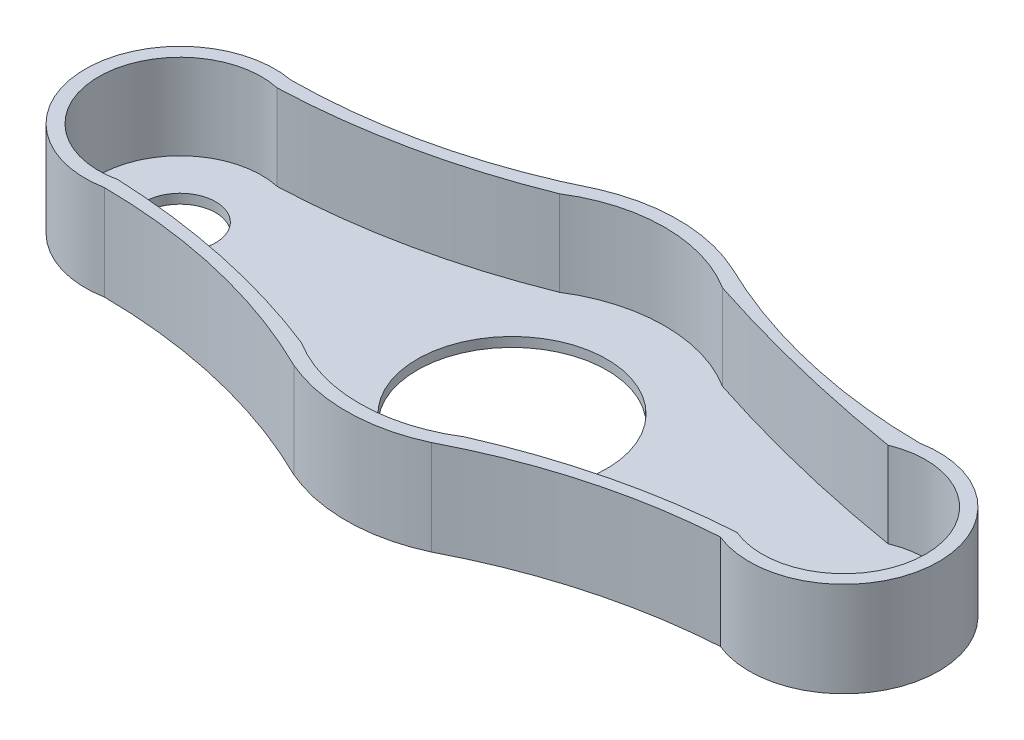
ISO-10303-21;
HEADER;
FILE_DESCRIPTION(('STEP AP214'),'2;1');
FILE_NAME('part.step','',(''),(''),'','','');
FILE_SCHEMA(('AUTOMOTIVE_DESIGN { 1 0 10303 214 1 1 1 1 }'));
ENDSEC;
DATA;
#1=APPLICATION_CONTEXT('core data for automotive mechanical design processes');
#2=APPLICATION_PROTOCOL_DEFINITION('international standard','automotive_design',2000,#1);
#3=PRODUCT_CONTEXT('',#1,'mechanical');
#4=PRODUCT('Part','Part','',(#3));
#5=PRODUCT_RELATED_PRODUCT_CATEGORY('part','',(#4));
#6=PRODUCT_DEFINITION_FORMATION('','',#4);
#7=PRODUCT_DEFINITION_CONTEXT('part definition',#1,'design');
#8=PRODUCT_DEFINITION('design','',#6,#7);
#9=PRODUCT_DEFINITION_SHAPE('','',#8);
#10=(LENGTH_UNIT() NAMED_UNIT(*) SI_UNIT(.MILLI.,.METRE.));
#11=(NAMED_UNIT(*) PLANE_ANGLE_UNIT() SI_UNIT($,.RADIAN.));
#12=(NAMED_UNIT(*) SI_UNIT($,.STERADIAN.) SOLID_ANGLE_UNIT());
#13=UNCERTAINTY_MEASURE_WITH_UNIT(LENGTH_MEASURE(1.E-05),#10,'distance_accuracy_value','');
#14=(GEOMETRIC_REPRESENTATION_CONTEXT(3) GLOBAL_UNCERTAINTY_ASSIGNED_CONTEXT((#13)) GLOBAL_UNIT_ASSIGNED_CONTEXT((#10,
#11,#12)) REPRESENTATION_CONTEXT('',''));
#15=CARTESIAN_POINT('',(0.,0.,0.));
#16=DIRECTION('',(0.,0.,1.));
#17=DIRECTION('',(1.,0.,0.));
#18=AXIS2_PLACEMENT_3D('',#15,#16,#17);
#19=CARTESIAN_POINT('',(-3.70941284252284,20.,0.));
#20=DIRECTION('',(0.,-1.,0.));
#21=DIRECTION('',(0.,0.,-1.));
#22=AXIS2_PLACEMENT_3D('',#19,#20,#21);
#23=CYLINDRICAL_SURFACE('',#22,7.5);
#24=CARTESIAN_POINT('',(-3.70941284252284,0.,0.));
#25=DIRECTION('',(0.,1.,0.));
#26=DIRECTION('',(0.,0.,1.));
#27=AXIS2_PLACEMENT_3D('',#24,#25,#26);
#28=CIRCLE('',#27,7.5);
#29=CARTESIAN_POINT('',(-3.70941284252284,0.,7.5));
#30=VERTEX_POINT('',#29);
#31=EDGE_CURVE('E197',#30,#30,#28,.T.);
#32=ORIENTED_EDGE('',*,*,#31,.F.);
#33=EDGE_LOOP('',(#32));
#34=FACE_BOUND('',#33,.T.);
#35=CARTESIAN_POINT('',(-3.70941284252284,2.,0.));
#36=DIRECTION('',(0.,1.,0.));
#37=DIRECTION('',(0.,0.,1.));
#38=AXIS2_PLACEMENT_3D('',#35,#36,#37);
#39=CIRCLE('',#38,7.5);
#40=CARTESIAN_POINT('',(-3.70941284252284,2.,7.5));
#41=VERTEX_POINT('',#40);
#42=EDGE_CURVE('E193',#41,#41,#39,.T.);
#43=ORIENTED_EDGE('',*,*,#42,.T.);
#44=EDGE_LOOP('',(#43));
#45=FACE_BOUND('',#44,.T.);
#46=ADVANCED_FACE('F41',(#34,#45),#23,.F.);
#47=CARTESIAN_POINT('',(136.290587157477,20.,0.));
#48=DIRECTION('',(0.,-1.,0.));
#49=DIRECTION('',(0.,0.,-1.));
#50=AXIS2_PLACEMENT_3D('',#47,#48,#49);
#51=CYLINDRICAL_SURFACE('',#50,7.50000000000001);
#52=CARTESIAN_POINT('',(136.290587157477,0.,0.));
#53=DIRECTION('',(0.,1.,0.));
#54=DIRECTION('',(0.,0.,1.));
#55=AXIS2_PLACEMENT_3D('',#52,#53,#54);
#56=CIRCLE('',#55,7.50000000000001);
#57=CARTESIAN_POINT('',(136.290587157477,0.,7.50000000000001));
#58=VERTEX_POINT('',#57);
#59=EDGE_CURVE('E192',#58,#58,#56,.T.);
#60=ORIENTED_EDGE('',*,*,#59,.F.);
#61=EDGE_LOOP('',(#60));
#62=FACE_BOUND('',#61,.T.);
#63=CARTESIAN_POINT('',(136.290587157477,2.,0.));
#64=DIRECTION('',(0.,1.,0.));
#65=DIRECTION('',(0.,0.,1.));
#66=AXIS2_PLACEMENT_3D('',#63,#64,#65);
#67=CIRCLE('',#66,7.50000000000001);
#68=CARTESIAN_POINT('',(136.290587157477,2.,7.50000000000001));
#69=VERTEX_POINT('',#68);
#70=EDGE_CURVE('E225',#69,#69,#67,.T.);
#71=ORIENTED_EDGE('',*,*,#70,.T.);
#72=EDGE_LOOP('',(#71));
#73=FACE_BOUND('',#72,.T.);
#74=ADVANCED_FACE('F210',(#62,#73),#51,.F.);
#75=CARTESIAN_POINT('',(66.2905871574772,20.,0.));
#76=DIRECTION('',(0.,-1.,0.));
#77=DIRECTION('',(0.,0.,-1.));
#78=AXIS2_PLACEMENT_3D('',#75,#76,#77);
#79=CYLINDRICAL_SURFACE('',#78,20.);
#80=CARTESIAN_POINT('',(66.2905871574772,0.,0.));
#81=DIRECTION('',(0.,1.,0.));
#82=DIRECTION('',(0.,0.,1.));
#83=AXIS2_PLACEMENT_3D('',#80,#81,#82);
#84=CIRCLE('',#83,20.);
#85=CARTESIAN_POINT('',(66.2905871574772,0.,20.));
#86=VERTEX_POINT('',#85);
#87=EDGE_CURVE('E189',#86,#86,#84,.T.);
#88=ORIENTED_EDGE('',*,*,#87,.F.);
#89=EDGE_LOOP('',(#88));
#90=FACE_BOUND('',#89,.T.);
#91=CARTESIAN_POINT('',(66.2905871574772,2.,0.));
#92=DIRECTION('',(0.,1.,0.));
#93=DIRECTION('',(0.,0.,1.));
#94=AXIS2_PLACEMENT_3D('',#91,#92,#93);
#95=CIRCLE('',#94,20.);
#96=CARTESIAN_POINT('',(66.2905871574772,2.,20.));
#97=VERTEX_POINT('',#96);
#98=EDGE_CURVE('E44',#97,#97,#95,.T.);
#99=ORIENTED_EDGE('',*,*,#98,.T.);
#100=EDGE_LOOP('',(#99));
#101=FACE_BOUND('',#100,.T.);
#102=ADVANCED_FACE('F43',(#90,#101),#79,.F.);
#103=CARTESIAN_POINT('',(133.534659461397,20.,-139.649207998908));
#104=DIRECTION('',(0.,-1.,0.));
#105=DIRECTION('',(0.,0.,-1.));
#106=AXIS2_PLACEMENT_3D('',#103,#104,#105);
#107=CYLINDRICAL_SURFACE('',#106,120.);
#108=CARTESIAN_POINT('',(133.534659461397,0.,-139.649207998908));
#109=DIRECTION('',(0.,1.,0.));
#110=DIRECTION('',(0.,0.,1.));
#111=AXIS2_PLACEMENT_3D('',#108,#109,#110);
#112=CIRCLE('',#111,120.);
#113=CARTESIAN_POINT('',(81.0387041699493,0.,-31.7410309313738));
#114=VERTEX_POINT('',#113);
#115=CARTESIAN_POINT('',(132.581174314954,0.,-19.6529961167178));
#116=VERTEX_POINT('',#115);
#117=EDGE_CURVE('E168',#114,#116,#112,.T.);
#118=ORIENTED_EDGE('',*,*,#117,.F.);
#119=DIRECTION('',(0.,-1.,0.));
#120=VECTOR('',#119,1.);
#121=CARTESIAN_POINT('',(81.0387041699493,20.,-31.7410309313738));
#122=LINE('',#121,#120);
#123=CARTESIAN_POINT('',(81.0387041699493,20.,-31.7410309313738));
#124=VERTEX_POINT('',#123);
#125=EDGE_CURVE('E11',#124,#114,#122,.T.);
#126=ORIENTED_EDGE('',*,*,#125,.F.);
#127=CARTESIAN_POINT('',(133.534659461397,20.,-139.649207998908));
#128=DIRECTION('',(0.,1.,0.));
#129=DIRECTION('',(0.,0.,1.));
#130=AXIS2_PLACEMENT_3D('',#127,#128,#129);
#131=CIRCLE('',#130,120.);
#132=CARTESIAN_POINT('',(132.581174314954,20.,-19.6529961167178));
#133=VERTEX_POINT('',#132);
#134=EDGE_CURVE('E190',#124,#133,#131,.T.);
#135=ORIENTED_EDGE('',*,*,#134,.T.);
#136=DIRECTION('',(0.,-1.,0.));
#137=VECTOR('',#136,1.);
#138=CARTESIAN_POINT('',(132.581174314954,20.,-19.6529961167178));
#139=LINE('',#138,#137);
#140=EDGE_CURVE('E98',#133,#116,#139,.T.);
#141=ORIENTED_EDGE('',*,*,#140,.T.);
#142=EDGE_LOOP('',(#118,#126,#135,#141));
#143=FACE_BOUND('',#142,.T.);
#144=ADVANCED_FACE('F200',(#143),#107,.F.);
#145=CARTESIAN_POINT('',(66.2905871574772,20.,0.));
#146=DIRECTION('',(0.,-1.,0.));
#147=DIRECTION('',(0.,0.,-1.));
#148=AXIS2_PLACEMENT_3D('',#145,#146,#147);
#149=CYLINDRICAL_SURFACE('',#148,35.);
#150=CARTESIAN_POINT('',(66.2905871574772,0.,0.));
#151=DIRECTION('',(0.,1.,0.));
#152=DIRECTION('',(0.,0.,1.));
#153=AXIS2_PLACEMENT_3D('',#150,#151,#152);
#154=CIRCLE('',#153,35.);
#155=CARTESIAN_POINT('',(52.4479221513952,0.,-32.1462381240697));
#156=VERTEX_POINT('',#155);
#157=EDGE_CURVE('E167',#114,#156,#154,.T.);
#158=ORIENTED_EDGE('',*,*,#157,.T.);
#159=DIRECTION('',(0.,-1.,0.));
#160=VECTOR('',#159,1.);
#161=CARTESIAN_POINT('',(52.4479221513952,20.,-32.1462381240697));
#162=LINE('',#161,#160);
#163=CARTESIAN_POINT('',(52.4479221513952,20.,-32.1462381240697));
#164=VERTEX_POINT('',#163);
#165=EDGE_CURVE('E49',#164,#156,#162,.T.);
#166=ORIENTED_EDGE('',*,*,#165,.F.);
#167=CARTESIAN_POINT('',(66.2905871574772,20.,0.));
#168=DIRECTION('',(0.,1.,0.));
#169=DIRECTION('',(0.,0.,1.));
#170=AXIS2_PLACEMENT_3D('',#167,#168,#169);
#171=CIRCLE('',#170,35.);
#172=EDGE_CURVE('E228',#124,#164,#171,.T.);
#173=ORIENTED_EDGE('',*,*,#172,.F.);
#174=ORIENTED_EDGE('',*,*,#125,.T.);
#175=EDGE_LOOP('',(#158,#166,#173,#174));
#176=FACE_BOUND('',#175,.T.);
#177=ADVANCED_FACE('F170',(#176),#149,.T.);
#178=CARTESIAN_POINT('',(-0.871658411644109,20.,-139.649830290013));
#179=DIRECTION('',(0.,-1.,0.));
#180=DIRECTION('',(0.,0.,-1.));
#181=AXIS2_PLACEMENT_3D('',#178,#179,#180);
#182=CYLINDRICAL_SURFACE('',#181,120.);
#183=CARTESIAN_POINT('',(-0.871658411644109,0.,-139.649830290013));
#184=DIRECTION('',(0.,1.,0.));
#185=DIRECTION('',(0.,0.,1.));
#186=AXIS2_PLACEMENT_3D('',#183,#184,#185);
#187=CIRCLE('',#186,120.);
#188=CARTESIAN_POINT('',(0.,0.,-19.6529961167178));
#189=VERTEX_POINT('',#188);
#190=EDGE_CURVE('E161',#189,#156,#187,.T.);
#191=ORIENTED_EDGE('',*,*,#190,.F.);
#192=DIRECTION('',(0.,-1.,0.));
#193=VECTOR('',#192,1.);
#194=CARTESIAN_POINT('',(0.,20.,-19.6529961167178));
#195=LINE('',#194,#193);
#196=CARTESIAN_POINT('',(0.,20.,-19.6529961167178));
#197=VERTEX_POINT('',#196);
#198=EDGE_CURVE('E155',#197,#189,#195,.T.);
#199=ORIENTED_EDGE('',*,*,#198,.F.);
#200=CARTESIAN_POINT('',(-0.871658411644109,20.,-139.649830290013));
#201=DIRECTION('',(0.,1.,0.));
#202=DIRECTION('',(0.,0.,1.));
#203=AXIS2_PLACEMENT_3D('',#200,#201,#202);
#204=CIRCLE('',#203,120.);
#205=EDGE_CURVE('E162',#197,#164,#204,.T.);
#206=ORIENTED_EDGE('',*,*,#205,.T.);
#207=ORIENTED_EDGE('',*,*,#165,.T.);
#208=EDGE_LOOP('',(#191,#199,#206,#207));
#209=FACE_BOUND('',#208,.T.);
#210=ADVANCED_FACE('F157',(#209),#182,.F.);
#211=CARTESIAN_POINT('',(-3.70941284252284,20.,0.));
#212=DIRECTION('',(0.,-1.,0.));
#213=DIRECTION('',(0.,0.,-1.));
#214=AXIS2_PLACEMENT_3D('',#211,#212,#213);
#215=CYLINDRICAL_SURFACE('',#214,20.);
#216=CARTESIAN_POINT('',(-3.70941284252284,0.,0.));
#217=DIRECTION('',(0.,1.,0.));
#218=DIRECTION('',(0.,0.,1.));
#219=AXIS2_PLACEMENT_3D('',#216,#217,#218);
#220=CIRCLE('',#219,20.);
#221=CARTESIAN_POINT('',(0.,0.,19.6529961167178));
#222=VERTEX_POINT('',#221);
#223=EDGE_CURVE('E174',#189,#222,#220,.T.);
#224=ORIENTED_EDGE('',*,*,#223,.T.);
#225=DIRECTION('',(0.,-1.,0.));
#226=VECTOR('',#225,1.);
#227=CARTESIAN_POINT('',(0.,20.,19.6529961167178));
#228=LINE('',#227,#226);
#229=CARTESIAN_POINT('',(0.,20.,19.6529961167178));
#230=VERTEX_POINT('',#229);
#231=EDGE_CURVE('E144',#230,#222,#228,.T.);
#232=ORIENTED_EDGE('',*,*,#231,.F.);
#233=CARTESIAN_POINT('',(-3.70941284252284,20.,0.));
#234=DIRECTION('',(0.,1.,0.));
#235=DIRECTION('',(0.,0.,1.));
#236=AXIS2_PLACEMENT_3D('',#233,#234,#235);
#237=CIRCLE('',#236,20.);
#238=EDGE_CURVE('E235',#197,#230,#237,.T.);
#239=ORIENTED_EDGE('',*,*,#238,.F.);
#240=ORIENTED_EDGE('',*,*,#198,.T.);
#241=EDGE_LOOP('',(#224,#232,#239,#240));
#242=FACE_BOUND('',#241,.T.);
#243=ADVANCED_FACE('F240',(#242),#215,.T.);
#244=CARTESIAN_POINT('',(-0.871658411644109,20.,139.649830290013));
#245=DIRECTION('',(0.,-1.,0.));
#246=DIRECTION('',(0.,0.,-1.));
#247=AXIS2_PLACEMENT_3D('',#244,#245,#246);
#248=CYLINDRICAL_SURFACE('',#247,120.);
#249=CARTESIAN_POINT('',(-0.871658411644109,0.,139.649830290013));
#250=DIRECTION('',(0.,1.,0.));
#251=DIRECTION('',(0.,0.,1.));
#252=AXIS2_PLACEMENT_3D('',#249,#250,#251);
#253=CIRCLE('',#252,120.);
#254=CARTESIAN_POINT('',(52.4479221513952,0.,32.1462381240697));
#255=VERTEX_POINT('',#254);
#256=EDGE_CURVE('E180',#222,#255,#253,.F.);
#257=ORIENTED_EDGE('',*,*,#256,.T.);
#258=DIRECTION('',(0.,-1.,0.));
#259=VECTOR('',#258,1.);
#260=CARTESIAN_POINT('',(52.4479221513952,20.,32.1462381240697));
#261=LINE('',#260,#259);
#262=CARTESIAN_POINT('',(52.4479221513952,20.,32.1462381240697));
#263=VERTEX_POINT('',#262);
#264=EDGE_CURVE('E141',#263,#255,#261,.T.);
#265=ORIENTED_EDGE('',*,*,#264,.F.);
#266=CARTESIAN_POINT('',(-0.871658411644109,20.,139.649830290013));
#267=DIRECTION('',(0.,1.,0.));
#268=DIRECTION('',(0.,0.,1.));
#269=AXIS2_PLACEMENT_3D('',#266,#267,#268);
#270=CIRCLE('',#269,120.);
#271=EDGE_CURVE('E136',#230,#263,#270,.F.);
#272=ORIENTED_EDGE('',*,*,#271,.F.);
#273=ORIENTED_EDGE('',*,*,#231,.T.);
#274=EDGE_LOOP('',(#257,#265,#272,#273));
#275=FACE_BOUND('',#274,.T.);
#276=ADVANCED_FACE('F239',(#275),#248,.F.);
#277=CARTESIAN_POINT('',(66.2905871574772,20.,0.));
#278=DIRECTION('',(0.,-1.,0.));
#279=DIRECTION('',(0.,0.,-1.));
#280=AXIS2_PLACEMENT_3D('',#277,#278,#279);
#281=CYLINDRICAL_SURFACE('',#280,35.);
#282=CARTESIAN_POINT('',(66.2905871574772,0.,0.));
#283=DIRECTION('',(0.,1.,0.));
#284=DIRECTION('',(0.,0.,1.));
#285=AXIS2_PLACEMENT_3D('',#282,#283,#284);
#286=CIRCLE('',#285,35.);
#287=CARTESIAN_POINT('',(81.0387041699488,0.,31.7410309313741));
#288=VERTEX_POINT('',#287);
#289=EDGE_CURVE('E142',#255,#288,#286,.T.);
#290=ORIENTED_EDGE('',*,*,#289,.T.);
#291=DIRECTION('',(0.,-1.,0.));
#292=VECTOR('',#291,1.);
#293=CARTESIAN_POINT('',(81.0387041699488,20.,31.7410309313741));
#294=LINE('',#293,#292);
#295=CARTESIAN_POINT('',(81.0387041699488,20.,31.7410309313741));
#296=VERTEX_POINT('',#295);
#297=EDGE_CURVE('E130',#296,#288,#294,.T.);
#298=ORIENTED_EDGE('',*,*,#297,.F.);
#299=CARTESIAN_POINT('',(66.2905871574772,20.,0.));
#300=DIRECTION('',(0.,1.,0.));
#301=DIRECTION('',(0.,0.,1.));
#302=AXIS2_PLACEMENT_3D('',#299,#300,#301);
#303=CIRCLE('',#302,35.);
#304=EDGE_CURVE('E131',#263,#296,#303,.T.);
#305=ORIENTED_EDGE('',*,*,#304,.F.);
#306=ORIENTED_EDGE('',*,*,#264,.T.);
#307=EDGE_LOOP('',(#290,#298,#305,#306));
#308=FACE_BOUND('',#307,.T.);
#309=ADVANCED_FACE('F143',(#308),#281,.T.);
#310=CARTESIAN_POINT('',(136.261182192829,20.,138.279652665525));
#311=DIRECTION('',(0.,-1.,0.));
#312=DIRECTION('',(0.,0.,-1.));
#313=AXIS2_PLACEMENT_3D('',#310,#311,#312);
#314=CYLINDRICAL_SURFACE('',#313,120.);
#315=CARTESIAN_POINT('',(136.261182192829,0.,138.279652665525));
#316=DIRECTION('',(0.,1.,0.));
#317=DIRECTION('',(0.,0.,1.));
#318=AXIS2_PLACEMENT_3D('',#315,#316,#317);
#319=CIRCLE('',#318,120.);
#320=CARTESIAN_POINT('',(128.730725009447,0.,18.5161681862846));
#321=VERTEX_POINT('',#320);
#322=EDGE_CURVE('E184',#288,#321,#319,.F.);
#323=ORIENTED_EDGE('',*,*,#322,.T.);
#324=DIRECTION('',(0.,-1.,0.));
#325=VECTOR('',#324,1.);
#326=CARTESIAN_POINT('',(128.730725009447,20.,18.5161681862846));
#327=LINE('',#326,#325);
#328=CARTESIAN_POINT('',(128.730725009447,20.,18.5161681862846));
#329=VERTEX_POINT('',#328);
#330=EDGE_CURVE('E128',#329,#321,#327,.T.);
#331=ORIENTED_EDGE('',*,*,#330,.F.);
#332=CARTESIAN_POINT('',(136.261182192829,20.,138.279652665525));
#333=DIRECTION('',(0.,1.,0.));
#334=DIRECTION('',(0.,0.,1.));
#335=AXIS2_PLACEMENT_3D('',#332,#333,#334);
#336=CIRCLE('',#335,120.);
#337=EDGE_CURVE('E125',#296,#329,#336,.F.);
#338=ORIENTED_EDGE('',*,*,#337,.F.);
#339=ORIENTED_EDGE('',*,*,#297,.T.);
#340=EDGE_LOOP('',(#323,#331,#338,#339));
#341=FACE_BOUND('',#340,.T.);
#342=ADVANCED_FACE('F124',(#341),#314,.F.);
#343=CARTESIAN_POINT('',(136.290587157477,20.,0.));
#344=DIRECTION('',(0.,-1.,0.));
#345=DIRECTION('',(0.,0.,-1.));
#346=AXIS2_PLACEMENT_3D('',#343,#344,#345);
#347=CYLINDRICAL_SURFACE('',#346,20.);
#348=CARTESIAN_POINT('',(136.290587157477,0.,0.));
#349=DIRECTION('',(0.,1.,0.));
#350=DIRECTION('',(0.,0.,1.));
#351=AXIS2_PLACEMENT_3D('',#348,#349,#350);
#352=CIRCLE('',#351,20.);
#353=EDGE_CURVE('E186',#321,#116,#352,.T.);
#354=ORIENTED_EDGE('',*,*,#353,.T.);
#355=ORIENTED_EDGE('',*,*,#140,.F.);
#356=CARTESIAN_POINT('',(136.290587157477,20.,0.));
#357=DIRECTION('',(0.,1.,0.));
#358=DIRECTION('',(0.,0.,1.));
#359=AXIS2_PLACEMENT_3D('',#356,#357,#358);
#360=CIRCLE('',#359,20.);
#361=EDGE_CURVE('E66',#329,#133,#360,.T.);
#362=ORIENTED_EDGE('',*,*,#361,.F.);
#363=ORIENTED_EDGE('',*,*,#330,.T.);
#364=EDGE_LOOP('',(#354,#355,#362,#363));
#365=FACE_BOUND('',#364,.T.);
#366=ADVANCED_FACE('F278',(#365),#347,.T.);
#367=CARTESIAN_POINT('',(0.,20.,0.));
#368=DIRECTION('',(0.,1.,0.));
#369=DIRECTION('',(0.,0.,1.));
#370=AXIS2_PLACEMENT_3D('',#367,#368,#369);
#371=PLANE('',#370);
#372=CARTESIAN_POINT('',(-5.31541215485532,20.,-162.502071352585));
#373=DIRECTION('',(0.,-1.,0.));
#374=DIRECTION('',(0.,0.,1.));
#375=AXIS2_PLACEMENT_3D('',#372,#373,#374);
#376=CIRCLE('',#375,145.825985530963);
#377=CARTESIAN_POINT('',(49.0929141726461,20.,-27.2062765830624));
#378=VERTEX_POINT('',#377);
#379=CARTESIAN_POINT('',(0.,20.,-16.7729924091542));
#380=VERTEX_POINT('',#379);
#381=EDGE_CURVE('E60',#378,#380,#376,.T.);
#382=ORIENTED_EDGE('',*,*,#381,.F.);
#383=CARTESIAN_POINT('',(66.2905871574772,20.,0.));
#384=DIRECTION('',(0.,1.,0.));
#385=DIRECTION('',(0.,0.,1.));
#386=AXIS2_PLACEMENT_3D('',#383,#384,#385);
#387=CIRCLE('',#386,32.1860442056379);
#388=CARTESIAN_POINT('',(83.4882601423082,20.,-27.2062765830624));
#389=VERTEX_POINT('',#388);
#390=EDGE_CURVE('E429',#389,#378,#387,.T.);
#391=ORIENTED_EDGE('',*,*,#390,.F.);
#392=CARTESIAN_POINT('',(180.442862833766,20.,-324.098747389265));
#393=DIRECTION('',(0.,-1.,0.));
#394=DIRECTION('',(0.,0.,1.));
#395=AXIS2_PLACEMENT_3D('',#392,#393,#394);
#396=CIRCLE('',#395,312.322484308239);
#397=CARTESIAN_POINT('',(129.668226582917,20.,-15.9311460453466));
#398=VERTEX_POINT('',#397);
#399=EDGE_CURVE('E434',#398,#389,#396,.T.);
#400=ORIENTED_EDGE('',*,*,#399,.F.);
#401=CARTESIAN_POINT('',(136.290587157477,20.,0.));
#402=DIRECTION('',(0.,1.,0.));
#403=DIRECTION('',(0.,0.,1.));
#404=AXIS2_PLACEMENT_3D('',#401,#402,#403);
#405=CIRCLE('',#404,17.2527410546166);
#406=CARTESIAN_POINT('',(129.668226582917,20.,15.9311460453466));
#407=VERTEX_POINT('',#406);
#408=EDGE_CURVE('E464',#407,#398,#405,.T.);
#409=ORIENTED_EDGE('',*,*,#408,.F.);
#410=CARTESIAN_POINT('',(138.379406602824,20.,151.81790411005));
#411=DIRECTION('',(0.,-1.,0.));
#412=DIRECTION('',(0.,0.,-1.));
#413=AXIS2_PLACEMENT_3D('',#410,#411,#412);
#414=CIRCLE('',#413,136.16569198838);
#415=CARTESIAN_POINT('',(83.4882601423083,20.,27.2062765830624));
#416=VERTEX_POINT('',#415);
#417=EDGE_CURVE('E465',#416,#407,#414,.T.);
#418=ORIENTED_EDGE('',*,*,#417,.F.);
#419=CARTESIAN_POINT('',(66.2905871574772,20.,0.));
#420=DIRECTION('',(0.,1.,0.));
#421=DIRECTION('',(0.,0.,1.));
#422=AXIS2_PLACEMENT_3D('',#419,#420,#421);
#423=CIRCLE('',#422,32.1860442056379);
#424=CARTESIAN_POINT('',(49.0929141726461,20.,27.2062765830624));
#425=VERTEX_POINT('',#424);
#426=EDGE_CURVE('E459',#425,#416,#423,.T.);
#427=ORIENTED_EDGE('',*,*,#426,.F.);
#428=CARTESIAN_POINT('',(-6.443566603327,20.,167.810504305155));
#429=DIRECTION('',(0.,-1.,0.));
#430=DIRECTION('',(0.,0.,-1.));
#431=AXIS2_PLACEMENT_3D('',#428,#429,#430);
#432=CIRCLE('',#431,151.174897222741);
#433=CARTESIAN_POINT('',(0.,20.,16.7729924091542));
#434=VERTEX_POINT('',#433);
#435=EDGE_CURVE('E457',#434,#425,#432,.T.);
#436=ORIENTED_EDGE('',*,*,#435,.F.);
#437=CARTESIAN_POINT('',(-3.70941284252284,20.,0.));
#438=DIRECTION('',(0.,1.,0.));
#439=DIRECTION('',(0.,0.,1.));
#440=AXIS2_PLACEMENT_3D('',#437,#438,#439);
#441=CIRCLE('',#440,17.1782716823846);
#442=EDGE_CURVE('E452',#380,#434,#441,.T.);
#443=ORIENTED_EDGE('',*,*,#442,.F.);
#444=EDGE_LOOP('',(#382,#391,#400,#409,#418,#427,#436,#443));
#445=FACE_BOUND('',#444,.T.);
#446=ORIENTED_EDGE('',*,*,#134,.F.);
#447=ORIENTED_EDGE('',*,*,#172,.T.);
#448=ORIENTED_EDGE('',*,*,#205,.F.);
#449=ORIENTED_EDGE('',*,*,#238,.T.);
#450=ORIENTED_EDGE('',*,*,#271,.T.);
#451=ORIENTED_EDGE('',*,*,#304,.T.);
#452=ORIENTED_EDGE('',*,*,#337,.T.);
#453=ORIENTED_EDGE('',*,*,#361,.T.);
#454=EDGE_LOOP('',(#446,#447,#448,#449,#450,#451,#452,#453));
#455=FACE_BOUND('',#454,.T.);
#456=ADVANCED_FACE('F133',(#445,#455),#371,.T.);
#457=CARTESIAN_POINT('',(0.,0.,0.));
#458=DIRECTION('',(0.,1.,0.));
#459=DIRECTION('',(0.,0.,1.));
#460=AXIS2_PLACEMENT_3D('',#457,#458,#459);
#461=PLANE('',#460);
#462=ORIENTED_EDGE('',*,*,#87,.T.);
#463=EDGE_LOOP('',(#462));
#464=FACE_BOUND('',#463,.T.);
#465=ORIENTED_EDGE('',*,*,#59,.T.);
#466=EDGE_LOOP('',(#465));
#467=FACE_BOUND('',#466,.T.);
#468=ORIENTED_EDGE('',*,*,#31,.T.);
#469=EDGE_LOOP('',(#468));
#470=FACE_BOUND('',#469,.T.);
#471=ORIENTED_EDGE('',*,*,#117,.T.);
#472=ORIENTED_EDGE('',*,*,#353,.F.);
#473=ORIENTED_EDGE('',*,*,#322,.F.);
#474=ORIENTED_EDGE('',*,*,#289,.F.);
#475=ORIENTED_EDGE('',*,*,#256,.F.);
#476=ORIENTED_EDGE('',*,*,#223,.F.);
#477=ORIENTED_EDGE('',*,*,#190,.T.);
#478=ORIENTED_EDGE('',*,*,#157,.F.);
#479=EDGE_LOOP('',(#471,#472,#473,#474,#475,#476,#477,#478));
#480=FACE_BOUND('',#479,.T.);
#481=ADVANCED_FACE('F172',(#464,#467,#470,#480),#461,.F.);
#482=CARTESIAN_POINT('',(-5.31541215485532,2.,-162.502071352585));
#483=DIRECTION('',(0.,1.,0.));
#484=DIRECTION('',(0.,0.,1.));
#485=AXIS2_PLACEMENT_3D('',#482,#483,#484);
#486=CYLINDRICAL_SURFACE('',#485,145.825985530963);
#487=ORIENTED_EDGE('',*,*,#381,.T.);
#488=DIRECTION('',(0.,1.,0.));
#489=VECTOR('',#488,1.);
#490=CARTESIAN_POINT('',(0.,2.,-16.7729924091542));
#491=LINE('',#490,#489);
#492=CARTESIAN_POINT('',(0.,2.,-16.7729924091542));
#493=VERTEX_POINT('',#492);
#494=EDGE_CURVE('E451',#493,#380,#491,.T.);
#495=ORIENTED_EDGE('',*,*,#494,.F.);
#496=CARTESIAN_POINT('',(-5.31541215485532,2.,-162.502071352585));
#497=DIRECTION('',(0.,-1.,0.));
#498=DIRECTION('',(0.,0.,1.));
#499=AXIS2_PLACEMENT_3D('',#496,#497,#498);
#500=CIRCLE('',#499,145.825985530963);
#501=CARTESIAN_POINT('',(49.0929141726461,2.,-27.2062765830624));
#502=VERTEX_POINT('',#501);
#503=EDGE_CURVE('E423',#502,#493,#500,.T.);
#504=ORIENTED_EDGE('',*,*,#503,.F.);
#505=DIRECTION('',(0.,1.,0.));
#506=VECTOR('',#505,1.);
#507=CARTESIAN_POINT('',(49.0929141726461,2.,-27.2062765830624));
#508=LINE('',#507,#506);
#509=EDGE_CURVE('E469',#502,#378,#508,.T.);
#510=ORIENTED_EDGE('',*,*,#509,.T.);
#511=EDGE_LOOP('',(#487,#495,#504,#510));
#512=FACE_BOUND('',#511,.T.);
#513=ADVANCED_FACE('F308',(#512),#486,.T.);
#514=CARTESIAN_POINT('',(66.2905871574772,2.,0.));
#515=DIRECTION('',(0.,1.,0.));
#516=DIRECTION('',(0.,0.,1.));
#517=AXIS2_PLACEMENT_3D('',#514,#515,#516);
#518=CYLINDRICAL_SURFACE('',#517,32.1860442056379);
#519=ORIENTED_EDGE('',*,*,#390,.T.);
#520=ORIENTED_EDGE('',*,*,#509,.F.);
#521=CARTESIAN_POINT('',(66.2905871574772,2.,0.));
#522=DIRECTION('',(0.,1.,0.));
#523=DIRECTION('',(0.,0.,1.));
#524=AXIS2_PLACEMENT_3D('',#521,#522,#523);
#525=CIRCLE('',#524,32.1860442056379);
#526=CARTESIAN_POINT('',(83.4882601423082,2.,-27.2062765830624));
#527=VERTEX_POINT('',#526);
#528=EDGE_CURVE('E428',#527,#502,#525,.T.);
#529=ORIENTED_EDGE('',*,*,#528,.F.);
#530=DIRECTION('',(0.,1.,0.));
#531=VECTOR('',#530,1.);
#532=CARTESIAN_POINT('',(83.4882601423082,2.,-27.2062765830624));
#533=LINE('',#532,#531);
#534=EDGE_CURVE('E472',#527,#389,#533,.T.);
#535=ORIENTED_EDGE('',*,*,#534,.T.);
#536=EDGE_LOOP('',(#519,#520,#529,#535));
#537=FACE_BOUND('',#536,.T.);
#538=ADVANCED_FACE('F328',(#537),#518,.F.);
#539=CARTESIAN_POINT('',(180.442862833766,2.,-324.098747389265));
#540=DIRECTION('',(0.,1.,0.));
#541=DIRECTION('',(0.,0.,1.));
#542=AXIS2_PLACEMENT_3D('',#539,#540,#541);
#543=CYLINDRICAL_SURFACE('',#542,312.322484308239);
#544=ORIENTED_EDGE('',*,*,#399,.T.);
#545=ORIENTED_EDGE('',*,*,#534,.F.);
#546=CARTESIAN_POINT('',(180.442862833766,2.,-324.098747389265));
#547=DIRECTION('',(0.,-1.,0.));
#548=DIRECTION('',(0.,0.,1.));
#549=AXIS2_PLACEMENT_3D('',#546,#547,#548);
#550=CIRCLE('',#549,312.322484308239);
#551=CARTESIAN_POINT('',(129.668226582917,2.,-15.9311460453466));
#552=VERTEX_POINT('',#551);
#553=EDGE_CURVE('E447',#552,#527,#550,.T.);
#554=ORIENTED_EDGE('',*,*,#553,.F.);
#555=DIRECTION('',(0.,1.,0.));
#556=VECTOR('',#555,1.);
#557=CARTESIAN_POINT('',(129.668226582917,2.,-15.9311460453466));
#558=LINE('',#557,#556);
#559=EDGE_CURVE('E474',#552,#398,#558,.T.);
#560=ORIENTED_EDGE('',*,*,#559,.T.);
#561=EDGE_LOOP('',(#544,#545,#554,#560));
#562=FACE_BOUND('',#561,.T.);
#563=ADVANCED_FACE('F337',(#562),#543,.T.);
#564=CARTESIAN_POINT('',(136.290587157477,2.,0.));
#565=DIRECTION('',(0.,1.,0.));
#566=DIRECTION('',(0.,0.,1.));
#567=AXIS2_PLACEMENT_3D('',#564,#565,#566);
#568=CYLINDRICAL_SURFACE('',#567,17.2527410546166);
#569=ORIENTED_EDGE('',*,*,#408,.T.);
#570=ORIENTED_EDGE('',*,*,#559,.F.);
#571=CARTESIAN_POINT('',(136.290587157477,2.,0.));
#572=DIRECTION('',(0.,1.,0.));
#573=DIRECTION('',(0.,0.,1.));
#574=AXIS2_PLACEMENT_3D('',#571,#572,#573);
#575=CIRCLE('',#574,17.2527410546166);
#576=CARTESIAN_POINT('',(129.668226582917,2.,15.9311460453466));
#577=VERTEX_POINT('',#576);
#578=EDGE_CURVE('E443',#577,#552,#575,.T.);
#579=ORIENTED_EDGE('',*,*,#578,.F.);
#580=DIRECTION('',(0.,1.,0.));
#581=VECTOR('',#580,1.);
#582=CARTESIAN_POINT('',(129.668226582917,2.,15.9311460453466));
#583=LINE('',#582,#581);
#584=EDGE_CURVE('E476',#577,#407,#583,.T.);
#585=ORIENTED_EDGE('',*,*,#584,.T.);
#586=EDGE_LOOP('',(#569,#570,#579,#585));
#587=FACE_BOUND('',#586,.T.);
#588=ADVANCED_FACE('F346',(#587),#568,.F.);
#589=CARTESIAN_POINT('',(138.379406602824,2.,151.81790411005));
#590=DIRECTION('',(0.,1.,0.));
#591=DIRECTION('',(0.,0.,1.));
#592=AXIS2_PLACEMENT_3D('',#589,#590,#591);
#593=CYLINDRICAL_SURFACE('',#592,136.16569198838);
#594=ORIENTED_EDGE('',*,*,#417,.T.);
#595=ORIENTED_EDGE('',*,*,#584,.F.);
#596=CARTESIAN_POINT('',(138.379406602824,2.,151.81790411005));
#597=DIRECTION('',(0.,-1.,0.));
#598=DIRECTION('',(0.,0.,-1.));
#599=AXIS2_PLACEMENT_3D('',#596,#597,#598);
#600=CIRCLE('',#599,136.16569198838);
#601=CARTESIAN_POINT('',(83.4882601423083,2.,27.2062765830624));
#602=VERTEX_POINT('',#601);
#603=EDGE_CURVE('E445',#602,#577,#600,.T.);
#604=ORIENTED_EDGE('',*,*,#603,.F.);
#605=DIRECTION('',(0.,1.,0.));
#606=VECTOR('',#605,1.);
#607=CARTESIAN_POINT('',(83.4882601423083,2.,27.2062765830624));
#608=LINE('',#607,#606);
#609=EDGE_CURVE('E481',#602,#416,#608,.T.);
#610=ORIENTED_EDGE('',*,*,#609,.T.);
#611=EDGE_LOOP('',(#594,#595,#604,#610));
#612=FACE_BOUND('',#611,.T.);
#613=ADVANCED_FACE('F357',(#612),#593,.T.);
#614=CARTESIAN_POINT('',(66.2905871574772,2.,0.));
#615=DIRECTION('',(0.,1.,0.));
#616=DIRECTION('',(0.,0.,1.));
#617=AXIS2_PLACEMENT_3D('',#614,#615,#616);
#618=CYLINDRICAL_SURFACE('',#617,32.1860442056379);
#619=ORIENTED_EDGE('',*,*,#426,.T.);
#620=ORIENTED_EDGE('',*,*,#609,.F.);
#621=CARTESIAN_POINT('',(66.2905871574772,2.,0.));
#622=DIRECTION('',(0.,1.,0.));
#623=DIRECTION('',(0.,0.,1.));
#624=AXIS2_PLACEMENT_3D('',#621,#622,#623);
#625=CIRCLE('',#624,32.1860442056379);
#626=CARTESIAN_POINT('',(49.0929141726461,2.,27.2062765830624));
#627=VERTEX_POINT('',#626);
#628=EDGE_CURVE('E438',#627,#602,#625,.T.);
#629=ORIENTED_EDGE('',*,*,#628,.F.);
#630=DIRECTION('',(0.,1.,0.));
#631=VECTOR('',#630,1.);
#632=CARTESIAN_POINT('',(49.0929141726461,2.,27.2062765830624));
#633=LINE('',#632,#631);
#634=EDGE_CURVE('E482',#627,#425,#633,.T.);
#635=ORIENTED_EDGE('',*,*,#634,.T.);
#636=EDGE_LOOP('',(#619,#620,#629,#635));
#637=FACE_BOUND('',#636,.T.);
#638=ADVANCED_FACE('F366',(#637),#618,.F.);
#639=CARTESIAN_POINT('',(-6.443566603327,2.,167.810504305155));
#640=DIRECTION('',(0.,1.,0.));
#641=DIRECTION('',(0.,0.,1.));
#642=AXIS2_PLACEMENT_3D('',#639,#640,#641);
#643=CYLINDRICAL_SURFACE('',#642,151.174897222741);
#644=ORIENTED_EDGE('',*,*,#435,.T.);
#645=ORIENTED_EDGE('',*,*,#634,.F.);
#646=CARTESIAN_POINT('',(-6.443566603327,2.,167.810504305155));
#647=DIRECTION('',(0.,-1.,0.));
#648=DIRECTION('',(0.,0.,-1.));
#649=AXIS2_PLACEMENT_3D('',#646,#647,#648);
#650=CIRCLE('',#649,151.174897222741);
#651=CARTESIAN_POINT('',(0.,2.,16.7729924091542));
#652=VERTEX_POINT('',#651);
#653=EDGE_CURVE('E435',#652,#627,#650,.T.);
#654=ORIENTED_EDGE('',*,*,#653,.F.);
#655=DIRECTION('',(0.,1.,0.));
#656=VECTOR('',#655,1.);
#657=CARTESIAN_POINT('',(0.,2.,16.7729924091542));
#658=LINE('',#657,#656);
#659=EDGE_CURVE('E490',#652,#434,#658,.T.);
#660=ORIENTED_EDGE('',*,*,#659,.T.);
#661=EDGE_LOOP('',(#644,#645,#654,#660));
#662=FACE_BOUND('',#661,.T.);
#663=ADVANCED_FACE('F378',(#662),#643,.T.);
#664=CARTESIAN_POINT('',(-3.70941284252284,2.,0.));
#665=DIRECTION('',(0.,1.,0.));
#666=DIRECTION('',(0.,0.,1.));
#667=AXIS2_PLACEMENT_3D('',#664,#665,#666);
#668=CYLINDRICAL_SURFACE('',#667,17.1782716823846);
#669=ORIENTED_EDGE('',*,*,#442,.T.);
#670=ORIENTED_EDGE('',*,*,#659,.F.);
#671=CARTESIAN_POINT('',(-3.70941284252284,2.,0.));
#672=DIRECTION('',(0.,1.,0.));
#673=DIRECTION('',(0.,0.,1.));
#674=AXIS2_PLACEMENT_3D('',#671,#672,#673);
#675=CIRCLE('',#674,17.1782716823846);
#676=EDGE_CURVE('E422',#493,#652,#675,.T.);
#677=ORIENTED_EDGE('',*,*,#676,.F.);
#678=ORIENTED_EDGE('',*,*,#494,.T.);
#679=EDGE_LOOP('',(#669,#670,#677,#678));
#680=FACE_BOUND('',#679,.T.);
#681=ADVANCED_FACE('F389',(#680),#668,.F.);
#682=CARTESIAN_POINT('',(30.4875875013109,2.,-81.2510356762924));
#683=DIRECTION('',(0.,1.,0.));
#684=DIRECTION('',(0.,0.,1.));
#685=AXIS2_PLACEMENT_3D('',#682,#683,#684);
#686=PLANE('',#685);
#687=ORIENTED_EDGE('',*,*,#42,.F.);
#688=EDGE_LOOP('',(#687));
#689=FACE_BOUND('',#688,.T.);
#690=ORIENTED_EDGE('',*,*,#70,.F.);
#691=EDGE_LOOP('',(#690));
#692=FACE_BOUND('',#691,.T.);
#693=ORIENTED_EDGE('',*,*,#98,.F.);
#694=EDGE_LOOP('',(#693));
#695=FACE_BOUND('',#694,.T.);
#696=ORIENTED_EDGE('',*,*,#503,.T.);
#697=ORIENTED_EDGE('',*,*,#676,.T.);
#698=ORIENTED_EDGE('',*,*,#653,.T.);
#699=ORIENTED_EDGE('',*,*,#628,.T.);
#700=ORIENTED_EDGE('',*,*,#603,.T.);
#701=ORIENTED_EDGE('',*,*,#578,.T.);
#702=ORIENTED_EDGE('',*,*,#553,.T.);
#703=ORIENTED_EDGE('',*,*,#528,.T.);
#704=EDGE_LOOP('',(#696,#697,#698,#699,#700,#701,#702,#703));
#705=FACE_BOUND('',#704,.T.);
#706=ADVANCED_FACE('F397',(#689,#692,#695,#705),#686,.T.);
#707=CLOSED_SHELL('',(#46,#74,#102,#144,#177,#210,#243,#276,#309,#342,#366,#456,#481,#513,#538,
#563,#588,#613,#638,#663,#681,#706));
#708=MANIFOLD_SOLID_BREP('B2',#707);
#709=ADVANCED_BREP_SHAPE_REPRESENTATION('',(#18,#708),#14);
#710=SHAPE_DEFINITION_REPRESENTATION(#9,#709);
ENDSEC;
END-ISO-10303-21;
